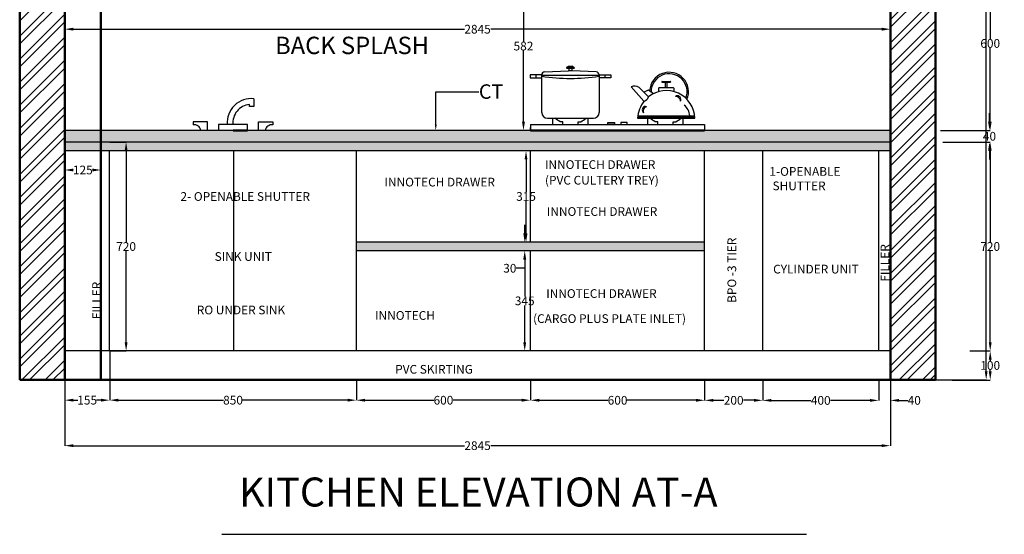
# Model space of a CAD drawing. Units: millimetres. Extents: x 26138 to 44889, y 15820 to 21179.
# Tile 3 of 8: x 31250 to 34642, y 15820 to 17594. Entities that reach past the tile are written whole.
import ezdxf
from ezdxf import colors
from ezdxf.entities.mleader import LeaderData, LeaderLine
from ezdxf.math import Vec2, Vec3

# ---------------------------------------------------------------- set-up
doc = ezdxf.new("R2010")
doc.units = ezdxf.units.MM
doc.header["$MEASUREMENT"] = 0
doc.header["$PDMODE"] = 3
for name, color, linetype, lineweight in [('A-ANNO-DIMS', 70, 'Continuous', 18), ('A-ANNO-TEXT', 7, 'Continuous', 18), ('A-ELEV', 7, 'Continuous', 25), ('A-FURN-PATT', 40, 'Continuous', 13), ('A-WALL', 1, 'Continuous', 50), ('A-WALL-PATT', 8, 'Continuous', 13)]:
    doc.layers.add(name, color=color, linetype=linetype, lineweight=lineweight)
doc.styles.get("Standard").update_dxf_attribs({"font": 'arial.ttf'})
doc.dimstyles.get("Standard").update_dxf_attribs({"dimtxt": 30, "dimasz": 30, "dimexe": 0.18, "dimexo": 0.0625, "dimgap": 0.09, "dimtad": 0, "dimtih": 1, "dimtoh": 1, "dimdec": 0, "dimzin": 0, "dimdsep": 46, "dimtxsty": 'Standard', "dimcen": 0.09, "dimadec": 0, "dimazin": 0, "dimtfac": 1, "dimtdec": 0, "dimtofl": 0, "dimtmove": 0, "dimatfit": 3, "dimfxl": 1, "dimtolj": 1, "dimtzin": 0, "dimarcsym": 0})
pattern_1 = [(45, (-3504.08, -2261.207), (-39.77476, 39.77476), []), (45, (-3477.56, -2261.207), (-39.77476, 39.77476), [])]

# ---------------------------------------------------------------- blocks, each defined once
blk = doc.blocks.new('*D48')
at = {"layer": 'A-ANNO-DIMS', "color": 0, "lineweight": -2, "transparency": 16777216}
for p, q in [((34523.2, 17812), (34594, 17812)), ((34593.8, 17782), (34593.8, 17527.4)), ((34593.8, 17242), (34593.8, 17496.6)), ((34422.5, 17212), (34594, 17212))]:
    blk.add_line(p, q, dxfattribs=at)
at = {"layer": 'A-ANNO-DIMS', "color": 0, "transparency": 16777216}
for points in [[(34588.8, 17782), (34598.8, 17782), (34593.8, 17812)], [(34588.8, 17242), (34598.8, 17242), (34593.8, 17212)]]:
    blk.add_solid(points, dxfattribs=at)
at = {"layer": 'Defpoints', "color": 0, "transparency": 16777216}
for p in [(34523.1, 17812), (34422.5, 17212), (34593.8, 17212)]:
    blk.add_point(p, dxfattribs=at)
at = {"layer": 'A-ANNO-DIMS', "color": 0, "transparency": 16777216, "insert": (34593.8, 17512), "char_height": 30, "attachment_point": 5}
blk.add_mtext('\\A1;600', dxfattribs=at)
blk = doc.blocks.new('*D49')
at = {"layer": 'A-ANNO-DIMS', "color": 0, "lineweight": -2, "transparency": 16777216}
for p, q in [((34591.3, 17242), (34591.3, 17272)), ((34523.2, 17212), (34591.5, 17212)), ((34523.2, 17172), (34591.5, 17172)), ((34591.3, 17142), (34591.3, 17112))]:
    blk.add_line(p, q, dxfattribs=at)
at = {"layer": 'A-ANNO-DIMS', "color": 0, "transparency": 16777216}
for points in [[(34586.3, 17242), (34596.3, 17242), (34591.3, 17212)], [(34586.3, 17142), (34596.3, 17142), (34591.3, 17172)]]:
    blk.add_solid(points, dxfattribs=at)
at = {"layer": 'Defpoints', "color": 0, "transparency": 16777216}
for p in [(34523.1, 17212), (34523.1, 17172), (34591.3, 17172)]:
    blk.add_point(p, dxfattribs=at)
at = {"layer": 'A-ANNO-DIMS', "color": 0, "transparency": 16777216, "insert": (34591.3, 17192), "char_height": 30, "attachment_point": 5}
blk.add_mtext('\\A1;40', dxfattribs=at)
blk = doc.blocks.new('*D50')
at = {"layer": 'A-ANNO-DIMS', "color": 0, "lineweight": -2, "transparency": 16777216}
for p, q in [((34430.6, 17172), (34594, 17172)), ((34593.8, 17142), (34593.8, 16827.4)), ((34593.8, 16482), (34593.8, 16796.6)), ((34523.2, 16452), (34594, 16452))]:
    blk.add_line(p, q, dxfattribs=at)
at = {"layer": 'A-ANNO-DIMS', "color": 0, "transparency": 16777216}
for points in [[(34588.8, 17142), (34598.8, 17142), (34593.8, 17172)], [(34588.8, 16482), (34598.8, 16482), (34593.8, 16452)]]:
    blk.add_solid(points, dxfattribs=at)
at = {"layer": 'Defpoints', "color": 0, "transparency": 16777216}
for p in [(34430.5, 17172), (34523.1, 16452), (34593.8, 16452)]:
    blk.add_point(p, dxfattribs=at)
at = {"layer": 'A-ANNO-DIMS', "color": 0, "transparency": 16777216, "insert": (34593.8, 16812), "char_height": 30, "attachment_point": 5}
blk.add_mtext('\\A1;720', dxfattribs=at)
blk = doc.blocks.new('*D51')
at = {"layer": 'A-ANNO-DIMS', "color": 0, "lineweight": -2, "transparency": 16777216}
for p, q in [((34523.2, 16452), (34594, 16452)), ((34593.8, 16422), (34593.8, 16417.3)), ((34593.8, 16381.7), (34593.8, 16386.5)), ((34463.2, 16351.7), (34594, 16351.7))]:
    blk.add_line(p, q, dxfattribs=at)
at = {"layer": 'A-ANNO-DIMS', "color": 0, "transparency": 16777216}
for points in [[(34588.8, 16422), (34598.8, 16422), (34593.8, 16452)], [(34588.8, 16381.7), (34598.8, 16381.7), (34593.8, 16351.7)]]:
    blk.add_solid(points, dxfattribs=at)
at = {"layer": 'Defpoints', "color": 0, "transparency": 16777216}
for p in [(34523.1, 16452), (34463.1, 16351.7), (34593.8, 16351.7)]:
    blk.add_point(p, dxfattribs=at)
at = {"layer": 'A-ANNO-DIMS', "color": 0, "transparency": 16777216, "insert": (34593.8, 16401.9), "char_height": 30, "attachment_point": 5}
blk.add_mtext('\\A1;100', dxfattribs=at)
blk = doc.blocks.new('*D56')
at = {"layer": 'A-ANNO-DIMS', "color": 0, "lineweight": -2, "transparency": 16777216}
for p, q in [((31559.9, 16451.9), (31559.9, 16282.1)), ((31404.9, 16351.9), (31404.9, 16282.1)), ((31434.9, 16282.3), (31450.4, 16282.3)), ((31529.9, 16282.3), (31514.3, 16282.3))]:
    blk.add_line(p, q, dxfattribs=at)
at = {"layer": 'A-ANNO-DIMS', "color": 0, "transparency": 16777216}
for points in [[(31434.9, 16287.3), (31434.9, 16277.3), (31404.9, 16282.3)], [(31529.9, 16287.3), (31529.9, 16277.3), (31559.9, 16282.3)]]:
    blk.add_solid(points, dxfattribs=at)
at = {"layer": 'Defpoints', "color": 0, "transparency": 16777216}
for p in [(31559.9, 16452), (31404.9, 16352), (31559.9, 16282.3)]:
    blk.add_point(p, dxfattribs=at)
at = {"layer": 'A-ANNO-DIMS', "color": 0, "transparency": 16777216, "insert": (31482.4, 16282.3), "char_height": 30, "attachment_point": 5}
blk.add_mtext('\\A1;155', dxfattribs=at)
blk = doc.blocks.new('*D57')
at = {"layer": 'A-ANNO-DIMS', "color": 0, "lineweight": -2, "transparency": 16777216}
for p, q in [((31559.9, 16351.9), (31559.9, 16282.1)), ((32409.9, 16351.9), (32409.9, 16282.1)), ((31589.9, 16282.3), (31951.7, 16282.3)), ((32379.9, 16282.3), (32018.1, 16282.3))]:
    blk.add_line(p, q, dxfattribs=at)
at = {"layer": 'A-ANNO-DIMS', "color": 0, "transparency": 16777216}
for points in [[(31589.9, 16287.3), (31589.9, 16277.3), (31559.9, 16282.3)], [(32379.9, 16287.3), (32379.9, 16277.3), (32409.9, 16282.3)]]:
    blk.add_solid(points, dxfattribs=at)
at = {"layer": 'Defpoints', "color": 0, "transparency": 16777216}
for p in [(31559.9, 16352), (32409.9, 16352), (32409.9, 16282.3)]:
    blk.add_point(p, dxfattribs=at)
at = {"layer": 'A-ANNO-DIMS', "color": 0, "transparency": 16777216, "insert": (31984.9, 16282.3), "char_height": 30, "attachment_point": 5}
blk.add_mtext('\\A1;850', dxfattribs=at)
blk = doc.blocks.new('*D58')
at = {"layer": 'A-ANNO-DIMS', "color": 0, "lineweight": -2, "transparency": 16777216}
for p, q in [((32409.9, 16351.9), (32409.9, 16281.9)), ((33009.9, 16351.9), (33009.9, 16281.9)), ((32439.9, 16282.1), (32676.6, 16282.1)), ((32979.9, 16282.1), (32743.1, 16282.1))]:
    blk.add_line(p, q, dxfattribs=at)
at = {"layer": 'A-ANNO-DIMS', "color": 0, "transparency": 16777216}
for points in [[(32439.9, 16287.1), (32439.9, 16277.1), (32409.9, 16282.1)], [(32979.9, 16287.1), (32979.9, 16277.1), (33009.9, 16282.1)]]:
    blk.add_solid(points, dxfattribs=at)
at = {"layer": 'Defpoints', "color": 0, "transparency": 16777216}
for p in [(32409.9, 16352), (33009.9, 16352), (33009.9, 16282.1)]:
    blk.add_point(p, dxfattribs=at)
at = {"layer": 'A-ANNO-DIMS', "color": 0, "transparency": 16777216, "insert": (32709.9, 16282.1), "char_height": 30, "attachment_point": 5}
blk.add_mtext('\\A1;600', dxfattribs=at)
blk = doc.blocks.new('*D59')
at = {"layer": 'A-ANNO-DIMS', "color": 0, "lineweight": -2, "transparency": 16777216}
for p, q in [((33009.9, 16351.9), (33009.9, 16281.7)), ((33609.9, 16351.9), (33609.9, 16281.7)), ((33039.9, 16281.9), (33276.6, 16281.9)), ((33579.9, 16281.9), (33343.1, 16281.9))]:
    blk.add_line(p, q, dxfattribs=at)
at = {"layer": 'A-ANNO-DIMS', "color": 0, "transparency": 16777216}
for points in [[(33039.9, 16286.9), (33039.9, 16276.9), (33009.9, 16281.9)], [(33579.9, 16286.9), (33579.9, 16276.9), (33609.9, 16281.9)]]:
    blk.add_solid(points, dxfattribs=at)
at = {"layer": 'Defpoints', "color": 0, "transparency": 16777216}
for p in [(33009.9, 16352), (33609.9, 16352), (33609.9, 16281.9)]:
    blk.add_point(p, dxfattribs=at)
at = {"layer": 'A-ANNO-DIMS', "color": 0, "transparency": 16777216, "insert": (33309.9, 16281.9), "char_height": 30, "attachment_point": 5}
blk.add_mtext('\\A1;600', dxfattribs=at)
blk = doc.blocks.new('*D60')
at = {"layer": 'A-ANNO-DIMS', "color": 0, "lineweight": -2, "transparency": 16777216}
for p, q in [((33609.9, 16351.9), (33609.9, 16281.5)), ((33809.9, 16351.9), (33809.9, 16281.5)), ((33639.9, 16281.7), (33676.4, 16281.7)), ((33779.9, 16281.7), (33743.3, 16281.7))]:
    blk.add_line(p, q, dxfattribs=at)
at = {"layer": 'A-ANNO-DIMS', "color": 0, "transparency": 16777216}
for points in [[(33639.9, 16286.7), (33639.9, 16276.7), (33609.9, 16281.7)], [(33779.9, 16286.7), (33779.9, 16276.7), (33809.9, 16281.7)]]:
    blk.add_solid(points, dxfattribs=at)
at = {"layer": 'Defpoints', "color": 0, "transparency": 16777216}
for p in [(33609.9, 16352), (33809.9, 16352), (33809.9, 16281.7)]:
    blk.add_point(p, dxfattribs=at)
at = {"layer": 'A-ANNO-DIMS', "color": 0, "transparency": 16777216, "insert": (33709.9, 16281.7), "char_height": 30, "attachment_point": 5}
blk.add_mtext('\\A1;200', dxfattribs=at)
blk = doc.blocks.new('*D61')
at = {"layer": 'A-ANNO-DIMS', "color": 0, "lineweight": -2, "transparency": 16777216}
for p, q in [((33809.9, 16351.9), (33809.9, 16281.4)), ((34209.9, 16351.9), (34209.9, 16281.4)), ((33839.9, 16281.5), (33976.1, 16281.5)), ((34179.9, 16281.5), (34043.6, 16281.5))]:
    blk.add_line(p, q, dxfattribs=at)
at = {"layer": 'A-ANNO-DIMS', "color": 0, "transparency": 16777216}
for points in [[(33839.9, 16286.5), (33839.9, 16276.5), (33809.9, 16281.5)], [(34179.9, 16286.5), (34179.9, 16276.5), (34209.9, 16281.5)]]:
    blk.add_solid(points, dxfattribs=at)
at = {"layer": 'Defpoints', "color": 0, "transparency": 16777216}
for p in [(33809.9, 16352), (34209.9, 16352), (34209.9, 16281.5)]:
    blk.add_point(p, dxfattribs=at)
at = {"layer": 'A-ANNO-DIMS', "color": 0, "transparency": 16777216, "insert": (34009.9, 16281.5), "char_height": 30, "attachment_point": 5}
blk.add_mtext('\\A1;400', dxfattribs=at)
blk = doc.blocks.new('*D62')
at = {"layer": 'A-ANNO-DIMS', "color": 0, "lineweight": -2, "transparency": 16777216}
for p, q in [((34209.9, 16351.9), (34209.9, 16281.4)), ((34249.9, 16351.9), (34249.9, 16281.4)), ((34179.9, 16281.5), (34149.9, 16281.5)), ((34279.9, 16281.5), (34309.9, 16281.5))]:
    blk.add_line(p, q, dxfattribs=at)
at = {"layer": 'A-ANNO-DIMS', "color": 0, "transparency": 16777216}
for points in [[(34179.9, 16286.5), (34179.9, 16276.5), (34209.9, 16281.5)], [(34279.9, 16286.5), (34279.9, 16276.5), (34249.9, 16281.5)]]:
    blk.add_solid(points, dxfattribs=at)
at = {"layer": 'Defpoints', "color": 0, "transparency": 16777216}
for p in [(34209.9, 16352), (34249.9, 16352), (34249.9, 16281.5)]:
    blk.add_point(p, dxfattribs=at)
at = {"layer": 'A-ANNO-DIMS', "color": 0, "transparency": 16777216, "insert": (34332, 16281.5), "char_height": 30, "attachment_point": 5}
blk.add_mtext('\\A1;40', dxfattribs=at)
blk = doc.blocks.new('*D63')
at = {"layer": 'A-ANNO-DIMS', "color": 0, "lineweight": -2, "transparency": 16777216}
for p, q in [((31404.9, 16352), (31404.9, 16125.2)), ((34249.9, 16352), (34249.9, 16125.2)), ((31434.9, 16125.4), (32782.1, 16125.4)), ((34219.9, 16125.4), (32872.6, 16125.4))]:
    blk.add_line(p, q, dxfattribs=at)
at = {"layer": 'A-ANNO-DIMS', "color": 0, "transparency": 16777216}
for points in [[(31434.9, 16130.4), (31434.9, 16120.4), (31404.9, 16125.4)], [(34219.9, 16130.4), (34219.9, 16120.4), (34249.9, 16125.4)]]:
    blk.add_solid(points, dxfattribs=at)
at = {"layer": 'Defpoints', "color": 0, "transparency": 16777216}
for p in [(31404.9, 16352), (34249.9, 16352), (34249.9, 16125.4)]:
    blk.add_point(p, dxfattribs=at)
at = {"layer": 'A-ANNO-DIMS', "color": 0, "transparency": 16777216, "insert": (32827.4, 16125.4), "char_height": 30, "attachment_point": 5}
blk.add_mtext('\\A1;2845', dxfattribs=at)
blk = doc.blocks.new('*D64')
at = {"layer": 'A-ANNO-DIMS', "color": 0, "lineweight": -2, "transparency": 16777216}
for p, q in [((33055.7, 17793.8), (32985.4, 17793.8)), ((32985.6, 17763.8), (32985.6, 17518.3)), ((32985.6, 17242), (32985.6, 17487.5)), ((33020.5, 17212), (32985.4, 17212))]:
    blk.add_line(p, q, dxfattribs=at)
at = {"layer": 'A-ANNO-DIMS', "color": 0, "transparency": 16777216}
for points in [[(32980.6, 17763.8), (32990.6, 17763.8), (32985.6, 17793.8)], [(32980.6, 17242), (32990.6, 17242), (32985.6, 17212)]]:
    blk.add_solid(points, dxfattribs=at)
at = {"layer": 'Defpoints', "color": 0, "transparency": 16777216}
for p in [(33055.8, 17793.8), (32985.6, 17212), (33020.5, 17212)]:
    blk.add_point(p, dxfattribs=at)
at = {"layer": 'A-ANNO-DIMS', "color": 0, "transparency": 16777216, "insert": (32985.6, 17502.9), "char_height": 30, "attachment_point": 5}
blk.add_mtext('\\A1;582', dxfattribs=at)
blk = doc.blocks.new('*D65')
at = {"layer": 'A-ANNO-DIMS', "color": 0, "lineweight": -2, "transparency": 16777216}
for p, q in [((31559.9, 17172), (31616.7, 17172)), ((31616.5, 17142), (31616.5, 16827.4)), ((31616.5, 16482), (31616.5, 16796.6)), ((31559.9, 16452), (31616.7, 16452))]:
    blk.add_line(p, q, dxfattribs=at)
at = {"layer": 'A-ANNO-DIMS', "color": 0, "transparency": 16777216}
for points in [[(31611.5, 17142), (31621.5, 17142), (31616.5, 17172)], [(31611.5, 16482), (31621.5, 16482), (31616.5, 16452)]]:
    blk.add_solid(points, dxfattribs=at)
at = {"layer": 'Defpoints', "color": 0, "transparency": 16777216}
for p in [(31559.9, 17172), (31616.5, 17172), (31559.9, 16452)]:
    blk.add_point(p, dxfattribs=at)
at = {"layer": 'A-ANNO-DIMS', "color": 0, "transparency": 16777216, "insert": (31616.5, 16812), "char_height": 30, "attachment_point": 5}
blk.add_mtext('\\A1;720', dxfattribs=at)
blk = doc.blocks.new('*D66')
at = {"layer": 'A-ANNO-DIMS', "color": 0, "lineweight": -2, "transparency": 16777216}
for p, q in [((33009.8, 17142), (32994.2, 17142)), ((32994.4, 17112), (32994.4, 16999.9)), ((32994.4, 16857), (32994.4, 16969.1)), ((33009.8, 16827), (32994.2, 16827))]:
    blk.add_line(p, q, dxfattribs=at)
at = {"layer": 'A-ANNO-DIMS', "color": 0, "transparency": 16777216}
for points in [[(32989.4, 17112), (32999.4, 17112), (32994.4, 17142)], [(32989.4, 16857), (32999.4, 16857), (32994.4, 16827)]]:
    blk.add_solid(points, dxfattribs=at)
at = {"layer": 'Defpoints', "color": 0, "transparency": 16777216}
for p in [(33009.9, 17142), (32994.4, 16827), (33009.9, 16827)]:
    blk.add_point(p, dxfattribs=at)
at = {"layer": 'A-ANNO-DIMS', "color": 0, "transparency": 16777216, "insert": (32994.4, 16984.5), "char_height": 30, "attachment_point": 5}
blk.add_mtext('\\A1;315', dxfattribs=at)
blk = doc.blocks.new('*D67')
at = {"layer": 'A-ANNO-DIMS', "color": 0, "lineweight": -2, "transparency": 16777216}
for p, q in [((32990.1, 16857), (32990.1, 16887)), ((33009.8, 16827), (32989.9, 16827)), ((33009.8, 16797), (32989.9, 16797)), ((32990.1, 16767), (32990.1, 16737)), ((32990.1, 16737), (32960.1, 16737))]:
    blk.add_line(p, q, dxfattribs=at)
at = {"layer": 'A-ANNO-DIMS', "color": 0, "transparency": 16777216}
for points in [[(32985.1, 16857), (32995.1, 16857), (32990.1, 16827)], [(32985.1, 16767), (32995.1, 16767), (32990.1, 16797)]]:
    blk.add_solid(points, dxfattribs=at)
at = {"layer": 'Defpoints', "color": 0, "transparency": 16777216}
for p in [(33009.9, 16827), (32990.1, 16797), (33009.9, 16797)]:
    blk.add_point(p, dxfattribs=at)
at = {"layer": 'A-ANNO-DIMS', "color": 0, "transparency": 16777216, "insert": (32938.6, 16737), "char_height": 30, "attachment_point": 5}
blk.add_mtext('\\A1;30', dxfattribs=at)
blk = doc.blocks.new('*D68')
at = {"layer": 'A-ANNO-DIMS', "color": 0, "lineweight": -2, "transparency": 16777216}
for p, q in [((33009.8, 16797), (32989.7, 16797)), ((32989.9, 16767), (32989.9, 16639.9)), ((32989.9, 16482), (32989.9, 16609.1)), ((33009.8, 16452), (32989.7, 16452))]:
    blk.add_line(p, q, dxfattribs=at)
at = {"layer": 'A-ANNO-DIMS', "color": 0, "transparency": 16777216}
for points in [[(32984.9, 16767), (32994.9, 16767), (32989.9, 16797)], [(32984.9, 16482), (32994.9, 16482), (32989.9, 16452)]]:
    blk.add_solid(points, dxfattribs=at)
at = {"layer": 'Defpoints', "color": 0, "transparency": 16777216}
for p in [(33009.9, 16797), (32989.9, 16452), (33009.9, 16452)]:
    blk.add_point(p, dxfattribs=at)
at = {"layer": 'A-ANNO-DIMS', "color": 0, "transparency": 16777216, "insert": (32989.9, 16624.5), "char_height": 30, "attachment_point": 5}
blk.add_mtext('\\A1;345', dxfattribs=at)
blk = doc.blocks.new('*D119')
at = {"layer": 'A-ANNO-DIMS', "color": 0, "lineweight": -2, "transparency": 16777216}
for p, q in [((31404.9, 17529.4), (31404.9, 17561.3)), ((31434.9, 17561.1), (32782.1, 17561.1)), ((34219.9, 17561.1), (32872.6, 17561.1)), ((34249.9, 17529.4), (34249.9, 17561.3))]:
    blk.add_line(p, q, dxfattribs=at)
at = {"layer": 'A-ANNO-DIMS', "color": 0, "transparency": 16777216}
for points in [[(31434.9, 17566.1), (31434.9, 17556.1), (31404.9, 17561.1)], [(34219.9, 17566.1), (34219.9, 17556.1), (34249.9, 17561.1)]]:
    blk.add_solid(points, dxfattribs=at)
at = {"layer": 'Defpoints', "color": 0, "transparency": 16777216}
for p in [(34249.9, 17561.1), (31404.9, 17529.3), (34249.9, 17529.3)]:
    blk.add_point(p, dxfattribs=at)
at = {"layer": 'A-ANNO-DIMS', "color": 0, "transparency": 16777216, "insert": (32827.4, 17561.1), "char_height": 30, "attachment_point": 5}
blk.add_mtext('\\A1;2845', dxfattribs=at)
blk = doc.blocks.new('*D122')
at = {"layer": 'A-ANNO-DIMS', "color": 0, "lineweight": -2, "transparency": 16777216}
for p, q in [((31404.9, 17141.9), (31404.9, 17075.5)), ((31529.9, 17141.9), (31529.9, 17075.5)), ((31434.9, 17075.7), (31435.4, 17075.7)), ((31499.9, 17075.7), (31499.3, 17075.7))]:
    blk.add_line(p, q, dxfattribs=at)
at = {"layer": 'A-ANNO-DIMS', "color": 0, "transparency": 16777216}
for points in [[(31434.9, 17080.7), (31434.9, 17070.7), (31404.9, 17075.7)], [(31499.9, 17080.7), (31499.9, 17070.7), (31529.9, 17075.7)]]:
    blk.add_solid(points, dxfattribs=at)
at = {"layer": 'Defpoints', "color": 0, "transparency": 16777216}
for p in [(31404.9, 17142), (31529.9, 17142), (31529.9, 17075.7)]:
    blk.add_point(p, dxfattribs=at)
at = {"layer": 'A-ANNO-DIMS', "color": 0, "transparency": 16777216, "insert": (31467.4, 17075.7), "char_height": 30, "attachment_point": 5}
blk.add_mtext('\\A1;125', dxfattribs=at)
blk = doc.blocks.new('*D137')
at = {"layer": 'A-ANNO-DIMS', "color": 0, "lineweight": -2, "transparency": 16777216}
for p, q in [((34404.9, 19102.3), (34580, 19102.3)), ((34579.9, 19072.3), (34579.9, 17742.6)), ((34579.9, 16382), (34579.9, 17711.8)), ((34404.9, 16352), (34580, 16352))]:
    blk.add_line(p, q, dxfattribs=at)
at = {"layer": 'A-ANNO-DIMS', "color": 0, "transparency": 16777216}
for points in [[(34574.9, 19072.3), (34584.9, 19072.3), (34579.9, 19102.3)], [(34574.9, 16382), (34584.9, 16382), (34579.9, 16352)]]:
    blk.add_solid(points, dxfattribs=at)
at = {"layer": 'Defpoints', "color": 0, "transparency": 16777216}
for p in [(34404.9, 19102.3), (34404.9, 16352), (34579.9, 16352)]:
    blk.add_point(p, dxfattribs=at)
at = {"layer": 'A-ANNO-DIMS', "color": 0, "transparency": 16777216, "insert": (34579.9, 17727.2), "char_height": 30, "attachment_point": 5}
blk.add_mtext('\\A1;2750.3', dxfattribs=at)

msp = doc.modelspace()

# ---------------------------------------------------------------- hatches: boundary and pattern name
at = {"layer": 'A-FURN-PATT'}
h = msp.add_hatch(color=256, dxfattribs=at)
h.dxf.hatch_style = 1
h.paths.add_polyline_path([(31404.861, 17172.011), (31404.861, 17142.011), (34249.859, 17142.011), (34249.859, 17172.011)])
h = msp.add_hatch(color=256, dxfattribs=at)
h.dxf.hatch_style = 1
h.paths.add_polyline_path([(33609.86, 16827.011), (32409.86, 16827.011), (32409.86, 16797.011), (33609.86, 16797.011)])
at = {"layer": 'A-WALL-PATT'}
h = msp.add_hatch(dxfattribs=at)
h.set_pattern_fill('ANSI32', color=256, scale=150)
h.set_pattern_definition(pattern_1)
h.paths.add_polyline_path([(31404.865, 19096.088), (31249.865, 19095.765), (31249.859, 16352.011), (31404.859, 16352.011)])
h = msp.add_hatch(dxfattribs=at)
h.set_pattern_fill('ANSI32', color=256, scale=150)
h.set_pattern_definition(pattern_1)
h.paths.add_polyline_path([(34404.859, 18942.01), (34249.859, 18942.01), (34249.859, 16352.011), (34404.859, 16352.011)])
h = msp.add_hatch(dxfattribs=at)
h.set_pattern_fill('AR-CONC', color=256, scale=4.9, angle=45)
h.set_pattern_definition([(95, (-3504.08, -2261.207), (27.026048, 22.677547), [3.675, -40.425]), (40, (-3504.08, -2261.207), (-30.869616, 21.25464), [2.94, -32.34]), (145.45144, (-3501.827, -2259.317), (-3.843568, 43.932186), [3.12327, -34.355963]), (91.1842, (-3511.01, -2254.277), (42.712976, 31.243075), [5.5125, -60.6375]), (141.63564, (-3507.45, -2251.674), (-1.367103, 66.13587), [4.68491, -51.533974]), (36.18416, (-3511.01, -2254.28), (-1.3671, 66.13587), [4.41, -48.51]), (66, (-3505.81, -2252.545), (34.631807, 6.731741), [3.675, -40.425]), (11, (-3505.81, -2252.545), (-16.69472, 33.555613), [2.94, -32.34]), (116.451445, (-3502.925, -2251.984), (17.937086, 40.287354), [3.12327, -34.355963]), (82.5, (-3504.079, -2261.207), (-11.112866, 11.955501), [0, -31.948, 0, -32.83, 0, -32.4625]), (52.5, (-3504.079, -2261.207), (-4.550774, 22.780563), [0, -18.718, 0, -31.213, 0, -12.3725]), (12.5, (-3511.805, -2268.934), (19.27749, 17.7145173), [0, -12.25, 0, -38.22, 0, -50.715]), (2.5, (-3515.27, -2272.398), (16.737909, 23.67483), [0, -15.925, 0, -25.382, 0, -36.015])])
h.paths.add_polyline_path([(34249.859, 17172.011), (34249.859, 17212.011), (31404.861, 17212.011), (31404.861, 17172.011)])

# ---------------------------------------------------------------- linework, layer by layer
at = {"layer": 'A-ELEV'}
for p, q in [((33048.4, 17403.804), (33008.4, 17403.804)), ((33008.4, 17403.804), (33008.4, 17393.804)), ((33028.4, 17403.804), (33028.4, 17393.804)), ((33048.4, 17273.804), (33048.4, 17403.804)), ((33048.4, 17403.804), (33048.4, 17403.804)), ((33058.4, 17413.804), (33140.964, 17417.649)), ((33133.97, 17426.354), (33160.871, 17426.354)), ((33133.97, 17426.354), (33133.97, 17426.354)), ((33138.97, 17431.354), (33138.97, 17431.424)), ((33138.97, 17431.354), (33155.871, 17431.354)), ((33153.876, 17417.649), (33140.964, 17417.649)), ((33140.97, 17433.424), (33153.871, 17433.424)), ((33236.441, 17413.804), (33153.876, 17417.649)), ((33155.871, 17431.354), (33155.871, 17431.424)), ((33160.871, 17426.354), (33160.871, 17426.354)), ((33246.441, 17403.804), (33246.441, 17273.804)), ((33246.441, 17403.804), (33286.441, 17403.804)), ((33246.441, 17403.804), (33246.441, 17403.804)), ((33266.441, 17403.804), (33266.441, 17393.804)), ((33286.441, 17403.804), (33286.441, 17393.804)), ((33008.4, 17393.804), (33048.4, 17393.804)), ((33048.4, 17402.454), (33246.441, 17402.454)), ((33286.441, 17393.804), (33246.441, 17393.804)), ((33462.492, 17379.771), (33462.492, 17378.771)), ((33462.492, 17378.771), (33492.354, 17378.771)), ((33463.492, 17380.771), (33491.354, 17380.771)), ((33474.423, 17359.537), (33474.423, 17378.771)), ((33480.423, 17359.537), (33480.423, 17378.771)), ((33492.354, 17379.771), (33492.354, 17378.771)), ((33357.217, 17362.012), (33400.709, 17312.789)), ((33416.44, 17328.138), (33384.3, 17360.277)), ((33400.37, 17344.208), (33416.907, 17352.034)), ((33416.907, 17352.034), (33433.686, 17339.04)), ((33451.531, 17345.831), (33451.531, 17357.537)), ((33453.531, 17359.537), (33501.315, 17359.537)), ((33503.315, 17357.576), (33503.543, 17345.87)), ((32057.147, 17321.181), (32057.147, 17294.141)), ((33400.709, 17312.789), (33401.253, 17313.269)), ((33509.447, 17328.712), (33511.777, 17331.161)), ((32041.442, 17294.141), (32041.539, 17301.434)), ((32057.147, 17294.141), (32041.442, 17294.141)), ((33409.422, 17293.688), (33406.367, 17295.134)), ((31897.393, 17241.276), (31847.664, 17241.276)), ((31847.664, 17241.276), (31847.664, 17231.258)), ((31897.393, 17211.276), (31897.393, 17241.276)), ((32072.325, 17211.276), (32072.325, 17241.276)), ((32072.325, 17241.276), (32122.054, 17241.276)), ((32122.054, 17241.276), (32122.054, 17231.258)), ((33068.4, 17253.804), (33226.441, 17253.804)), ((33086.705, 17232.011), (33086.705, 17253.804)), ((33208.136, 17232.011), (33208.136, 17253.804)), ((33378.805, 17253.912), (33576.412, 17253.912)), ((33378.955, 17256.912), (33576.251, 17256.912)), ((33379.197, 17259.912), (33575.998, 17259.912)), ((33379.531, 17262.912), (33575.654, 17262.912)), ((33414.373, 17232.011), (33414.373, 17253.804)), ((33535.804, 17232.011), (33535.804, 17253.804)), ((34249.859, 17212.011), (31404.859, 17212.011)), ((32034.859, 17232.011), (31934.859, 17232.011)), ((31934.859, 17232.011), (31934.859, 17212.011)), ((32034.859, 17212.011), (32034.859, 17232.011)), ((33009.861, 17232.011), (33609.861, 17232.011)), ((33009.861, 17232.011), (33009.861, 17212.011)), ((33009.861, 17212.011), (33009.861, 17222.011)), ((33174.096, 17232.011), (33208.136, 17232.011)), ((33501.765, 17232.011), (33535.804, 17232.011)), ((33609.861, 17232.011), (33609.861, 17212.011)), ((34249.859, 17172.011), (31404.859, 17172.011)), ((34249.859, 17142.011), (31404.859, 17142.011)), ((31559.859, 16452.011), (31559.861, 17142.011)), ((31986.398, 17142.011), (31986.398, 16452.011)), ((32409.859, 16452.011), (32409.861, 17142.01)), ((33009.86, 16827.011), (33009.861, 17142.008)), ((33609.859, 16452.011), (33609.861, 17142.007)), ((33809.859, 16452.011), (33809.861, 17142.007)), ((34209.859, 16452.011), (34209.861, 17142.006)), ((33609.86, 16827.011), (32409.86, 16827.011)), ((33609.86, 16797.011), (32409.86, 16797.011)), ((33009.859, 16452.011), (33009.86, 16797.011)), ((34249.859, 16452.011), (31404.859, 16452.011)), ((32409.859, 16352.009), (32409.859, 16352.011)), ((33609.859, 16352.006), (33609.859, 16352.011)), ((33809.859, 16352.006), (33809.859, 16352.011)), ((34209.859, 16352.005), (34209.859, 16352.011)), ((31946.635, 15819.809), (33960.312, 15819.809))]:
    msp.add_line(p, q, dxfattribs=at)
for points in [[(33139.559, 17426.354, -0.47928661), (33140.964, 17417.649)], [(33155.282, 17426.354, 0.47928661), (33153.876, 17417.649)], [(33120.744, 17232.011), (33120.744, 17241.407, 0.15287481), (33112.12, 17241.407, 0.01894931), (33093.421, 17253.804, -1.50829924)], [(33174.096, 17232.011), (33174.096, 17241.407, -0.15287481), (33182.721, 17241.407, -0.01894931), (33201.419, 17253.804, 1.50829924)], [(33448.413, 17232.011), (33448.413, 17241.407, 0.15287481), (33439.788, 17241.407, 0.01894931), (33421.09, 17253.804, -1.50829924)], [(33501.765, 17232.011), (33501.765, 17241.407, -0.15287481), (33510.389, 17241.407, -0.01894931), (33529.088, 17253.804, 1.50829924)]]:
    msp.add_lwpolyline(points, format="xyb", dxfattribs=at)
for points in [[(33298.754, 17232.011), (33276.54, 17232.011), (33276.54, 17239.988), (33298.754, 17239.988)], [(33320.964, 17232.011), (33343.178, 17232.011), (33343.178, 17239.988), (33320.964, 17239.988)]]:
    msp.add_lwpolyline(points, close=True, dxfattribs=at)
for centre, radius, start, end in [((33058.4, 17403.804), 10, 90, 180), ((33138.97, 17426.354), 5, 90, 180), ((33140.97, 17431.424), 2, 89.997317, 180), ((33153.871, 17431.424), 2, 0, 89.997317), ((33155.871, 17426.354), 5, 0, 90), ((33236.441, 17403.804), 10, 0, 90), ((33487.33, 17345.491), 67.034, 336.694061, 176.721438), ((33487.33, 17345.491), 62.034, 338.503343, 179.957077), ((33147.42, 18051.726), 660.446, 261.377147, 278.622853), ((33463.492, 17379.771), 1, 90, 180), ((33491.354, 17379.771), 1, 0, 90), ((33369.181, 17336.514), 28.165, 57.533932, 115.138947), ((33477.608, 17250.469), 98.864, 1.995689, 128.222327), ((33453.531, 17357.537), 2, 90, 180), ((33501.315, 17357.537), 2, 1.116074, 90), ((32047.627, 17238.613), 83.114, 83.423266, 184.556052), ((33477.608, 17250.469), 98.864, 140.563599, 178.004311), ((33396.209, 17333.136), 20.839, 282.469204, 346.123184), ((33510.874, 17312.962), 15.814, 1.141589, 95.175905), ((33515.264, 17318.913), 12.735, 333.734213, 105.895011), ((32047.627, 17238.613), 63.114, 95.535879, 186.004459), ((33068.4, 17273.804), 20, 180, 270), ((33226.441, 17273.804), 20, 270, 0), ((33407.525, 17282.451), 12.735, 95.214996, 227.375794), ((33413.764, 17278.481), 15.814, 105.934102, 199.968418), ((33507.496, 17258.937), 51.128, 4.458698, 51.456594), ((31851.583, 17209.609), 22, 6.267854, 100.261645), ((32118.135, 17209.609), 22, 79.738355, 173.732146)]:
    msp.add_arc(centre, radius, start, end, dxfattribs=at)
at = {"layer": 'A-WALL'}
for p, q in [((34404.859, 19102.334), (34404.859, 16352.011)), ((31249.859, 16352.011), (31249.865, 19096.349)), ((31404.859, 16352.011), (31404.865, 19096.348)), ((31529.859, 16352.011), (31529.865, 19096.348)), ((34249.859, 18942.01), (34249.859, 16352.011)), ((31984.859, 17212.011), (32034.859, 17212.011)), ((33009.861, 17212.011), (33609.861, 17212.011)), ((34404.859, 16352.011), (31249.859, 16352.011))]:
    msp.add_line(p, q, dxfattribs=at)

# ---------------------------------------------------------------- texts
at = {"layer": 'A-ANNO-TEXT'}
for s, height, p in [('BACK SPLASH', 60, (32129.917, 17475.142)), ('INNOTECH DRAWER', 30, (33059.756, 17079.424)), ('1-OPENABLE ', 30, (33832.949, 17055.683)), ('INNOTECH DRAWER', 30, (32506.859, 17018.991)), ('(PVC CULTERY TREY)', 30, (33059.756, 17025.466)), ('SHUTTER', 30, (33843.748, 17006.042)), ('2- OPENABLE SHUTTER', 30, (31803.875, 16969.336)), ('INNOTECH DRAWER', 30, (33066.236, 16917.551)), ('SINK UNIT', 30, (31921.616, 16762.447)), ('CYLINDER UNIT', 30, (33845.908, 16718.987)), ('INNOTECH DRAWER', 30, (33064.076, 16634.813)), ('RO UNDER SINK', 30, (31860.045, 16578.092)), ('INNOTECH', 30, (32474.462, 16559.273)), ('(CARGO PLUS PLATE INLET)', 30, (33018.721, 16548.481)), ('PVC SKIRTING', 30, (32543.575, 16373.659)), ('KITCHEN ELEVATION AT-A', 100, (32005.257, 15915.633))]:
    msp.add_text(s, height=height, dxfattribs=at).set_placement(p)
for s, p in [('BPO -3 TIER', (33718.482, 16617.547)), ('FILLER', (34246.099, 16690.879)), ('FILLER', (31529.859, 16561.31))]:
    msp.add_text(s, height=30, rotation=90, dxfattribs=at).set_placement(p)

# ---------------------------------------------------------------- dimensions: what is measured, and where the dimension line sits
at = {"layer": 'A-ANNO-DIMS'}
for base, p1, p2, override, picture, middle in [((34579.859, 16352.011), (34404.859, 19102.334), (34404.859, 16352.011), {"dimdec": 1, "dimlfac": 1, "dimrnd": 0, "dimzin": 0, "dimdsep": 46, "dimlunit": 2}, '*D137', (34579.859, 17727.172)), ((34593.789, 17212.011), (34523.108, 17812.011), (34422.485, 17212.011), {"dimclrd": 0, "dimclre": 0, "dimclrt": 0}, '*D48', (34593.789, 17512.011)), ((34591.289, 17172.011), (34523.108, 17212.011), (34523.108, 17172.011), {"dimclrd": 0, "dimclre": 0, "dimclrt": 0}, '*D49', (34591.289, 17192.011)), ((31616.516, 17172.011), (31559.86, 16452.011), (31559.861, 17172.011), {"dimclrd": 0, "dimclre": 0, "dimclrt": 0}, '*D65', (31616.516, 16812.011)), ((34593.789, 16452.011), (34430.532, 17172.011), (34523.108, 16452.011), {"dimclrd": 0, "dimclre": 0, "dimclrt": 0}, '*D50', (34593.789, 16812.011)), ((32994.411, 16827.008), (33009.861, 17142.008), (33009.861, 16827.008), {"dimclrd": 0, "dimclre": 0, "dimclrt": 0}, '*D66', (32994.411, 16984.508)), ((32990.103, 16797.008), (33009.861, 16827.008), (33009.861, 16797.008), {"dimclrd": 0, "dimclre": 0, "dimclrt": 0}, '*D67', (32938.587, 16737.008)), ((32989.923, 16452.008), (33009.861, 16797.008), (33009.861, 16452.008), {"dimclrd": 0, "dimclre": 0, "dimclrt": 0}, '*D68', (32989.923, 16624.508)), ((34593.789, 16351.747), (34523.108, 16452.011), (34463.147, 16351.747), {"dimclrd": 0, "dimclre": 0, "dimclrt": 0}, '*D51', (34593.789, 16401.879))]:
    dim = msp.add_linear_dim(base=base, p1=p1, p2=p2, angle=90, dimstyle='Standard', override=override, dxfattribs=at)
    dim.commit()
    dim.dimension.update_dxf_attribs({"geometry": picture, "text_midpoint": middle})
dim = msp.add_linear_dim(base=(32985.563, 17212.011), p1=(33055.779, 17793.785), p2=(33020.55, 17212.011), angle=90, dimstyle='Standard', override={"dimclrd": 0, "dimclre": 0, "dimclrt": 0}, dxfattribs=at)
dim.commit()
dim.dimension.update_dxf_attribs({"geometry": '*D64', "text_midpoint": (32985.563, 17502.898), "dimtype": 160})
for base, p1, p2, picture, middle in [((34249.859, 17561.099), (31404.861, 17529.327), (34249.859, 17529.327), '*D119', (32827.36, 17561.099)), ((31529.861, 17075.677), (31404.861, 17142.011), (31529.861, 17142.011), '*D122', (31467.361, 17075.677)), ((31559.859, 16282.266), (31404.859, 16352.011), (31559.859, 16452.011), '*D56', (31482.359, 16282.266)), ((34249.859, 16125.412), (31404.859, 16352.018), (34249.859, 16352.018), '*D63', (32827.359, 16125.412)), ((32409.859, 16282.266), (31559.859, 16352.011), (32409.859, 16352.011), '*D57', (31984.859, 16282.266)), ((33009.859, 16282.086), (32409.859, 16352.011), (33009.859, 16352.011), '*D58', (32709.859, 16282.086)), ((33609.859, 16281.906), (33009.859, 16352.011), (33609.859, 16352.011), '*D59', (33309.859, 16281.906)), ((33809.859, 16281.726), (33609.859, 16352.011), (33809.859, 16352.011), '*D60', (33709.859, 16281.726)), ((34209.859, 16281.546), (33809.859, 16352.011), (34209.859, 16352.011), '*D61', (34009.859, 16281.546)), ((34249.859, 16281.546), (34209.859, 16352.011), (34249.859, 16352.011), '*D62', (34331.988, 16281.546))]:
    dim = msp.add_linear_dim(base=base, p1=p1, p2=p2, dimstyle='Standard', override={"dimclrd": 0, "dimclre": 0, "dimclrt": 0}, dxfattribs=at)
    dim.commit()
    dim.dimension.update_dxf_attribs({"geometry": picture, "text_midpoint": middle})

# ---------------------------------------------------------------- leaders
at = {"layer": 'A-ANNO-TEXT'}
ml = msp.add_multileader_mtext('Standard', dxfattribs=at)
ml.set_content('CT', color=256)
ml.set_leader_properties()
ml.build(insert=Vec2(0, 0))
ml.multileader.update_dxf_attribs({"dogleg_length": 0.36, "arrow_head_size": 20})
ctx = ml.context
ctx.base_point, ctx.char_height, ctx.arrow_head_size, ctx.landing_gap_size, ctx.plane_origin = Vec3(32831.821, 17345.628), 50, 20, 0.09, Vec3(32831.461, 17345.628)
notes = []
notes.append((ctx, [(0, (1, 1, 0), (32831.461, 17345.628), (1, 0), 0.36, [(0, [(32683.431, 17211.811), (32683.431, 17345.628)], 0, [])])]))
ctx.mtext.insert, ctx.mtext.flow_direction = Vec3(32831.911, 17371.054), 5
for ctx, leaders in notes:
    for number, flags, end, landing, length, lines in leaders:
        leader = LeaderData()
        leader.index, (leader.has_last_leader_line, leader.has_dogleg_vector, leader.attachment_direction) = number, flags
        leader.last_leader_point, leader.dogleg_vector, leader.dogleg_length = Vec3(end), Vec3(landing), length
        for number, points, colour, breaks in lines:
            line = LeaderLine()
            line.index, line.vertices, line.color, line.breaks = number, Vec3.list(points), colors.encode_raw_color(colour), breaks
            leader.lines.append(line)
        ctx.leaders.append(leader)

doc.saveas('drawing.dxf')
